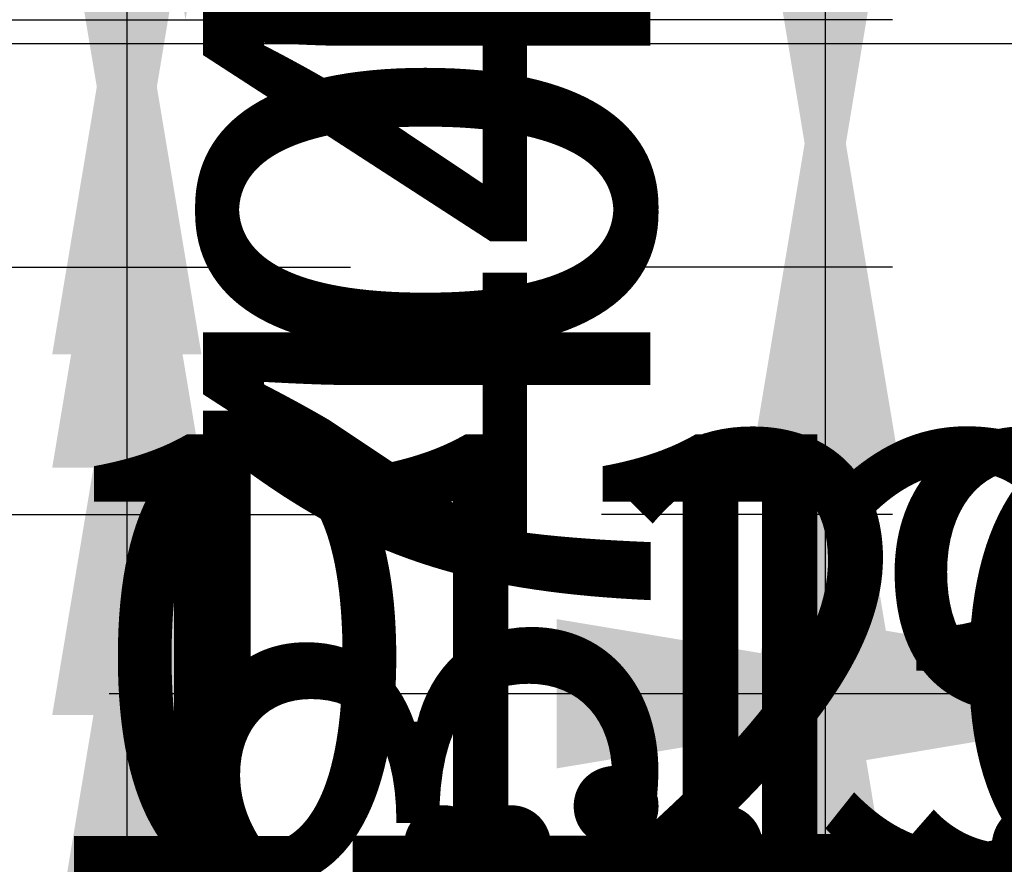
# Model space of a CAD drawing. Units: metres. Extents: x 782 to 1487, y 1262 to 7446.
# Tile 12 of 25: x 834.592 to 840.091, y 1288.353 to 1293.067. Entities that reach past the tile are written whole.
import ezdxf

# ---------------------------------------------------------------- set-up
doc = ezdxf.new("R2010")
doc.units = ezdxf.units.M
doc.layers.add('A-ANNO-DIMS', color=2, linetype='Continuous', lineweight=18)
doc.styles.get("Standard").update_dxf_attribs({"font": 'arial.ttf'})
doc.dimstyles.new('ISO-25', dxfattribs={"dimtxt": 2.5, "dimasz": 2.5, "dimexe": 1.25, "dimexo": 0.625, "dimtad": 1, "dimtxsty": 'Standard', "dimcen": 2.5, "dimadec": 0, "dimazin": 0, "dimtfac": 1, "dimtmove": 0, "dimatfit": 3, "dimfxl": 1, "dimarcsym": 0})

# ---------------------------------------------------------------- blocks, each defined once
blk = doc.blocks.new('*D6')
at = {"layer": 'A-ANNO-DIMS', "color": 0, "lineweight": -2, "transparency": 16777216}
for p, q in [((833.0375, 1307.3274), (836.7683, 1307.3274)), ((835.5183, 1304.8274), (835.5183, 1295.5674)), ((833.0375, 1293.0674), (836.7683, 1293.0674))]:
    blk.add_line(p, q, dxfattribs=at)
at = {"layer": 'A-ANNO-DIMS', "color": 0, "transparency": 16777216}
for points in [[(835.1017, 1304.8274), (835.935, 1304.8274), (835.5183, 1307.3274)], [(835.1017, 1295.5674), (835.935, 1295.5674), (835.5183, 1293.0674)]]:
    blk.add_solid(points, dxfattribs=at)
at = {"layer": 'Defpoints', "color": 0, "transparency": 16777216}
for p in [(832.4125, 1307.3274), (832.4125, 1293.0674), (835.5183, 1293.0674)]:
    blk.add_point(p, dxfattribs=at)
at = {"layer": 'A-ANNO-DIMS', "color": 0, "transparency": 16777216, "insert": (833.3909, 1300.1974), "char_height": 2.5, "attachment_point": 5, "rotation": 90}
blk.add_mtext('14,26', dxfattribs=at)
blk = doc.blocks.new('*D22')
at = {"layer": 'A-ANNO-DIMS', "color": 0, "lineweight": -2, "transparency": 16777216}
for p, q in [((812.7897, 1292.934), (810.2897, 1292.934)), ((815.2897, 1292.934), (816.1792, 1292.934)), ((818.6792, 1292.934), (848.8344, 1292.934)), ((815.2897, 1292.4424), (815.2897, 1291.684)), ((816.1792, 1292.4424), (816.1792, 1291.684))]:
    blk.add_line(p, q, dxfattribs=at)
at = {"layer": 'A-ANNO-DIMS', "color": 0, "transparency": 16777216}
for points in [[(812.7897, 1293.3507), (812.7897, 1292.5173), (815.2897, 1292.934)], [(818.6792, 1293.3507), (818.6792, 1292.5173), (816.1792, 1292.934)]]:
    blk.add_solid(points, dxfattribs=at)
at = {"layer": 'Defpoints', "color": 0, "transparency": 16777216}
for p in [(815.2897, 1293.0674), (816.1792, 1293.0674), (816.1792, 1292.934)]:
    blk.add_point(p, dxfattribs=at)
at = {"layer": 'A-ANNO-DIMS', "color": 0, "transparency": 16777216, "insert": (835.0068, 1294.8525), "char_height": 2.5, "attachment_point": 5}
blk.add_mtext('DOOR 0.89 TYP.', dxfattribs=at)
blk = doc.blocks.new('*D24')
at = {"layer": 'A-ANNO-DIMS', "color": 0, "lineweight": -2, "transparency": 16777216}
for p, q in [((811.2086, 1294.4231), (808.7086, 1294.4231)), ((813.7086, 1294.4231), (814.5592, 1294.4231)), ((817.0592, 1294.4231), (852.6493, 1294.4231)), ((813.7086, 1293.9257), (813.7086, 1293.1731)), ((814.5592, 1293.9257), (814.5592, 1293.1731))]:
    blk.add_line(p, q, dxfattribs=at)
at = {"layer": 'A-ANNO-DIMS', "color": 0, "transparency": 16777216}
for points in [[(811.2086, 1294.8398), (811.2086, 1294.0065), (813.7086, 1294.4231)], [(817.0592, 1294.8398), (817.0592, 1294.0065), (814.5592, 1294.4231)]]:
    blk.add_solid(points, dxfattribs=at)
at = {"layer": 'Defpoints', "color": 0, "transparency": 16777216}
for p in [(813.7086, 1294.5507), (814.5592, 1294.5507), (814.5592, 1294.4231)]:
    blk.add_point(p, dxfattribs=at)
at = {"layer": 'A-ANNO-DIMS', "color": 0, "transparency": 16777216, "insert": (836.1042, 1296.3416), "char_height": 2.5, "attachment_point": 5}
blk.add_mtext('DOOR D2 0.85 TYP.', dxfattribs=at)
blk = doc.blocks.new('*D87')
at = {"layer": 'A-ANNO-DIMS', "color": 0, "lineweight": -2, "transparency": 16777216}
for p, q in [((835.1905, 1309.8274), (835.1905, 1312.3274)), ((833.0375, 1307.3274), (836.4405, 1307.3274)), ((835.1905, 1307.3274), (835.1905, 1304.8669)), ((833.0382, 1304.8669), (836.4405, 1304.8669)), ((835.1905, 1302.3669), (835.1905, 1292.0821))]:
    blk.add_line(p, q, dxfattribs=at)
at = {"layer": 'A-ANNO-DIMS', "color": 0, "transparency": 16777216}
for points in [[(834.7738, 1309.8274), (835.6071, 1309.8274), (835.1905, 1307.3274)], [(834.7738, 1302.3669), (835.6071, 1302.3669), (835.1905, 1304.8669)]]:
    blk.add_solid(points, dxfattribs=at)
at = {"layer": 'Defpoints', "color": 0, "transparency": 16777216}
for p in [(832.4125, 1307.3274), (832.4132, 1304.8669), (835.1905, 1304.8669)]:
    blk.add_point(p, dxfattribs=at)
at = {"layer": 'A-ANNO-DIMS', "color": 0, "transparency": 16777216, "insert": (833.289, 1295.9745), "char_height": 2.5, "attachment_point": 5, "rotation": 90}
blk.add_mtext('2.46', dxfattribs=at)
blk = doc.blocks.new('*D88')
at = {"layer": 'A-ANNO-DIMS', "color": 0, "lineweight": -2, "transparency": 16777216}
for p, q in [((835.1905, 1307.3669), (835.1905, 1309.8669)), ((833.0382, 1304.8669), (836.4405, 1304.8669)), ((835.1905, 1304.8669), (835.1905, 1300.3378)), ((833.0381, 1300.3378), (836.4405, 1300.3378)), ((835.1905, 1297.8378), (835.1905, 1285.5459))]:
    blk.add_line(p, q, dxfattribs=at)
at = {"layer": 'A-ANNO-DIMS', "color": 0, "transparency": 16777216}
for points in [[(834.7738, 1307.3669), (835.6071, 1307.3669), (835.1905, 1304.8669)], [(834.7738, 1297.8378), (835.6071, 1297.8378), (835.1905, 1300.3378)]]:
    blk.add_solid(points, dxfattribs=at)
at = {"layer": 'Defpoints', "color": 0, "transparency": 16777216}
for p in [(832.4132, 1304.8669), (832.4131, 1300.3378), (835.1905, 1300.3378)]:
    blk.add_point(p, dxfattribs=at)
at = {"layer": 'A-ANNO-DIMS', "color": 0, "transparency": 16777216, "insert": (833.289, 1290.4419), "char_height": 2.5, "attachment_point": 5, "rotation": 90}
blk.add_mtext('4.529', dxfattribs=at)
blk = doc.blocks.new('*D89')
at = {"layer": 'A-ANNO-DIMS', "color": 0, "lineweight": -2, "transparency": 16777216}
for p, q in [((835.1905, 1302.8378), (835.1905, 1305.3378)), ((833.0381, 1300.3378), (836.4405, 1300.3378)), ((835.1905, 1300.3378), (835.1905, 1296.196)), ((833.0375, 1296.196), (836.4405, 1296.196)), ((835.1905, 1293.696), (835.1905, 1281.4347))]:
    blk.add_line(p, q, dxfattribs=at)
at = {"layer": 'A-ANNO-DIMS', "color": 0, "transparency": 16777216}
for points in [[(834.7738, 1302.8378), (835.6071, 1302.8378), (835.1905, 1300.3378)], [(834.7738, 1293.696), (835.6071, 1293.696), (835.1905, 1296.196)]]:
    blk.add_solid(points, dxfattribs=at)
at = {"layer": 'Defpoints', "color": 0, "transparency": 16777216}
for p in [(832.4131, 1300.3378), (832.4125, 1296.196), (835.1905, 1296.196)]:
    blk.add_point(p, dxfattribs=at)
at = {"layer": 'A-ANNO-DIMS', "color": 0, "transparency": 16777216, "insert": (833.3103, 1286.3153), "char_height": 2.5, "attachment_point": 5, "rotation": 90}
blk.add_mtext('4.142', dxfattribs=at)
blk = doc.blocks.new('*D90')
at = {"layer": 'A-ANNO-DIMS', "color": 0, "lineweight": -2, "transparency": 16777216}
for p, q in [((835.1905, 1298.696), (835.1905, 1301.196)), ((833.0375, 1296.196), (836.4405, 1296.196)), ((835.1905, 1296.196), (835.1905, 1293.6994)), ((833.0375, 1293.6994), (836.4405, 1293.6994)), ((835.1905, 1291.1994), (835.1905, 1280.9214))]:
    blk.add_line(p, q, dxfattribs=at)
at = {"layer": 'A-ANNO-DIMS', "color": 0, "transparency": 16777216}
for points in [[(834.7738, 1298.696), (835.6071, 1298.696), (835.1905, 1296.196)], [(834.7738, 1291.1994), (835.6071, 1291.1994), (835.1905, 1293.6994)]]:
    blk.add_solid(points, dxfattribs=at)
at = {"layer": 'Defpoints', "color": 0, "transparency": 16777216}
for p in [(832.4125, 1296.196), (832.4125, 1293.6994), (835.1905, 1293.6994)]:
    blk.add_point(p, dxfattribs=at)
at = {"layer": 'A-ANNO-DIMS', "color": 0, "transparency": 16777216, "insert": (833.289, 1284.8104), "char_height": 2.5, "attachment_point": 5, "rotation": 90}
blk.add_mtext('2.50', dxfattribs=at)
blk = doc.blocks.new('*D91')
at = {"layer": 'A-ANNO-DIMS', "color": 0, "lineweight": -2, "transparency": 16777216}
for p, q in [((835.1905, 1296.1994), (835.1905, 1298.6994)), ((833.0375, 1293.6994), (836.4405, 1293.6994)), ((835.1905, 1293.6994), (835.1905, 1293.0674)), ((833.0375, 1293.0674), (836.4405, 1293.0674)), ((835.1905, 1290.5674), (835.1905, 1278.4068))]:
    blk.add_line(p, q, dxfattribs=at)
at = {"layer": 'A-ANNO-DIMS', "color": 0, "transparency": 16777216}
for points in [[(834.7738, 1296.1994), (835.6071, 1296.1994), (835.1905, 1293.6994)], [(834.7738, 1290.5674), (835.6071, 1290.5674), (835.1905, 1293.0674)]]:
    blk.add_solid(points, dxfattribs=at)
at = {"layer": 'Defpoints', "color": 0, "transparency": 16777216}
for p in [(832.4125, 1293.6994), (832.4125, 1293.0674), (835.1905, 1293.0674)]:
    blk.add_point(p, dxfattribs=at)
at = {"layer": 'A-ANNO-DIMS', "color": 0, "transparency": 16777216, "insert": (833.2882, 1283.2371), "char_height": 2.5, "attachment_point": 5, "rotation": 90}
blk.add_mtext('0.632', dxfattribs=at)
blk = doc.blocks.new('*D92')
at = {"layer": 'A-ANNO-DIMS', "color": 0, "lineweight": -2, "transparency": 16777216}
for p, q in [((835.1905, 1295.5674), (835.1905, 1298.0674)), ((831.3406, 1293.0674), (836.4405, 1293.0674)), ((835.1905, 1293.0674), (835.1905, 1291.6863)), ((831.3406, 1291.6863), (836.4405, 1291.6863)), ((835.1905, 1289.1863), (835.1905, 1277.7181))]:
    blk.add_line(p, q, dxfattribs=at)
at = {"layer": 'A-ANNO-DIMS', "color": 0, "transparency": 16777216}
for points in [[(834.7738, 1295.5674), (835.6071, 1295.5674), (835.1905, 1293.0674)], [(834.7738, 1289.1863), (835.6071, 1289.1863), (835.1905, 1291.6863)]]:
    blk.add_solid(points, dxfattribs=at)
at = {"layer": 'Defpoints', "color": 0, "transparency": 16777216}
for p in [(830.7156, 1293.0674), (830.7156, 1291.6863), (835.1905, 1291.6863)]:
    blk.add_point(p, dxfattribs=at)
at = {"layer": 'A-ANNO-DIMS', "color": 0, "transparency": 16777216, "insert": (833.2882, 1282.2022), "char_height": 2.5, "attachment_point": 5, "rotation": 90}
blk.add_mtext('1.381', dxfattribs=at)
blk = doc.blocks.new('*D93')
at = {"layer": 'A-ANNO-DIMS', "color": 0, "lineweight": -2, "transparency": 16777216}
for p, q in [((835.1905, 1294.1863), (835.1905, 1296.6863)), ((831.3406, 1291.6863), (836.4405, 1291.6863)), ((835.1905, 1291.6863), (835.1905, 1290.3053)), ((831.3406, 1290.3053), (836.4405, 1290.3053)), ((835.1905, 1287.8053), (835.1905, 1276.337))]:
    blk.add_line(p, q, dxfattribs=at)
at = {"layer": 'A-ANNO-DIMS', "color": 0, "transparency": 16777216}
for points in [[(834.7738, 1294.1863), (835.6071, 1294.1863), (835.1905, 1291.6863)], [(834.7738, 1287.8053), (835.6071, 1287.8053), (835.1905, 1290.3053)]]:
    blk.add_solid(points, dxfattribs=at)
at = {"layer": 'Defpoints', "color": 0, "transparency": 16777216}
for p in [(830.7156, 1291.6863), (830.7156, 1290.3053), (835.1905, 1290.3053)]:
    blk.add_point(p, dxfattribs=at)
at = {"layer": 'A-ANNO-DIMS', "color": 0, "transparency": 16777216, "insert": (833.2882, 1280.8211), "char_height": 2.5, "attachment_point": 5, "rotation": 90}
blk.add_mtext('1.381', dxfattribs=at)
blk = doc.blocks.new('*D97')
at = {"layer": 'A-ANNO-DIMS', "color": 0, "lineweight": -2, "transparency": 16777216}
for p, q in [((827.9625, 1289.6803), (827.9625, 1286.0275)), ((829.1513, 1289.6803), (829.1513, 1286.0275)), ((825.4625, 1287.2775), (822.9625, 1287.2775)), ((827.9625, 1287.2775), (829.1513, 1287.2775)), ((831.6513, 1287.2775), (841.6649, 1287.2775))]:
    blk.add_line(p, q, dxfattribs=at)
at = {"layer": 'A-ANNO-DIMS', "color": 0, "transparency": 16777216}
for points in [[(825.4625, 1287.6941), (825.4625, 1286.8608), (827.9625, 1287.2775)], [(831.6513, 1287.6941), (831.6513, 1286.8608), (829.1513, 1287.2775)]]:
    blk.add_solid(points, dxfattribs=at)
at = {"layer": 'Defpoints', "color": 0, "transparency": 16777216}
for p in [(827.9625, 1290.3053), (829.1513, 1290.3053), (829.1513, 1287.2775)]:
    blk.add_point(p, dxfattribs=at)
at = {"layer": 'A-ANNO-DIMS', "color": 0, "transparency": 16777216, "insert": (837.9081, 1289.1789), "char_height": 2.5, "attachment_point": 5}
blk.add_mtext('1.19', dxfattribs=at)
blk = doc.blocks.new('*D98')
at = {"layer": 'A-ANNO-DIMS', "color": 0, "lineweight": -2, "transparency": 16777216}
for p, q in [((829.1513, 1289.6803), (829.1513, 1286.0275)), ((829.412, 1289.6803), (829.412, 1286.0275)), ((826.6513, 1287.2775), (824.1513, 1287.2775)), ((829.1513, 1287.2775), (829.412, 1287.2775)), ((831.912, 1287.2775), (842.1542, 1287.2775))]:
    blk.add_line(p, q, dxfattribs=at)
at = {"layer": 'A-ANNO-DIMS', "color": 0, "transparency": 16777216}
for points in [[(826.6513, 1287.6941), (826.6513, 1286.8608), (829.1513, 1287.2775)], [(831.912, 1287.6941), (831.912, 1286.8608), (829.412, 1287.2775)]]:
    blk.add_solid(points, dxfattribs=at)
at = {"layer": 'Defpoints', "color": 0, "transparency": 16777216}
for p in [(829.1513, 1290.3053), (829.412, 1290.3053), (829.412, 1287.2775)]:
    blk.add_point(p, dxfattribs=at)
at = {"layer": 'A-ANNO-DIMS', "color": 0, "transparency": 16777216, "insert": (838.2831, 1289.1789), "char_height": 2.5, "attachment_point": 5}
blk.add_mtext('0.26', dxfattribs=at)
blk = doc.blocks.new('*D99')
at = {"layer": 'A-ANNO-DIMS', "color": 0, "lineweight": -2, "transparency": 16777216}
for p, q in [((829.412, 1289.6803), (829.412, 1286.0275)), ((830.7156, 1289.6803), (830.7156, 1286.0275)), ((826.912, 1287.2775), (824.412, 1287.2775)), ((829.412, 1287.2775), (830.7156, 1287.2775)), ((833.2156, 1287.2775), (843.2156, 1287.2775))]:
    blk.add_line(p, q, dxfattribs=at)
at = {"layer": 'A-ANNO-DIMS', "color": 0, "transparency": 16777216}
for points in [[(826.912, 1287.6941), (826.912, 1286.8608), (829.412, 1287.2775)], [(833.2156, 1287.6941), (833.2156, 1286.8608), (830.7156, 1287.2775)]]:
    blk.add_solid(points, dxfattribs=at)
at = {"layer": 'Defpoints', "color": 0, "transparency": 16777216}
for p in [(829.412, 1290.3053), (830.7156, 1290.3053), (830.7156, 1287.2775)]:
    blk.add_point(p, dxfattribs=at)
at = {"layer": 'A-ANNO-DIMS', "color": 0, "transparency": 16777216, "insert": (839.4656, 1289.1798), "char_height": 2.5, "attachment_point": 5}
blk.add_mtext('1.30', dxfattribs=at)
blk = doc.blocks.new('*D100')
at = {"layer": 'A-ANNO-DIMS', "color": 0, "lineweight": -2, "transparency": 16777216}
for p, q in [((830.7156, 1289.6803), (830.7156, 1286.0275)), ((832.4125, 1289.6803), (832.4125, 1286.0275)), ((828.2156, 1287.2775), (825.7156, 1287.2775)), ((830.7156, 1287.2775), (832.4125, 1287.2775)), ((834.9125, 1287.2775), (846.8634, 1287.2775))]:
    blk.add_line(p, q, dxfattribs=at)
at = {"layer": 'A-ANNO-DIMS', "color": 0, "transparency": 16777216}
for points in [[(828.2156, 1287.6941), (828.2156, 1286.8608), (830.7156, 1287.2775)], [(834.9125, 1287.6941), (834.9125, 1286.8608), (832.4125, 1287.2775)]]:
    blk.add_solid(points, dxfattribs=at)
at = {"layer": 'Defpoints', "color": 0, "transparency": 16777216}
for p in [(830.7156, 1290.3053), (832.4125, 1290.3053), (832.4125, 1287.2775)]:
    blk.add_point(p, dxfattribs=at)
at = {"layer": 'A-ANNO-DIMS', "color": 0, "transparency": 16777216, "insert": (842.1379, 1289.1789), "char_height": 2.5, "attachment_point": 5}
blk.add_mtext('1.697', dxfattribs=at)
blk = doc.blocks.new('*D105')
at = {"layer": 'A-ANNO-DIMS', "color": 0, "lineweight": -2, "transparency": 16777216}
for p, q in [((840.0913, 1289.6803), (840.0913, 1288.0553)), ((841.2801, 1289.6803), (841.2801, 1288.0553)), ((837.5913, 1289.3053), (835.0913, 1289.3053)), ((840.0913, 1289.3053), (841.2801, 1289.3053)), ((843.7801, 1289.3053), (853.7938, 1289.3053))]:
    blk.add_line(p, q, dxfattribs=at)
at = {"layer": 'A-ANNO-DIMS', "color": 0, "transparency": 16777216}
for points in [[(837.5913, 1289.7219), (837.5913, 1288.8886), (840.0913, 1289.3053)], [(843.7801, 1289.7219), (843.7801, 1288.8886), (841.2801, 1289.3053)]]:
    blk.add_solid(points, dxfattribs=at)
at = {"layer": 'Defpoints', "color": 0, "transparency": 16777216}
for p in [(840.0913, 1290.3053), (841.2801, 1290.3053), (841.2801, 1289.3053)]:
    blk.add_point(p, dxfattribs=at)
at = {"layer": 'A-ANNO-DIMS', "color": 0, "transparency": 16777216, "insert": (850.037, 1291.2067), "char_height": 2.5, "attachment_point": 5}
blk.add_mtext('1.19', dxfattribs=at)
blk = doc.blocks.new('*D106')
at = {"layer": 'A-ANNO-DIMS', "color": 0, "lineweight": -2, "transparency": 16777216}
for p, q in [((841.2801, 1289.6803), (841.2801, 1288.0553)), ((841.5409, 1289.6803), (841.5409, 1288.0553)), ((838.7801, 1289.3053), (836.2801, 1289.3053)), ((841.2801, 1289.3053), (841.5409, 1289.3053)), ((844.0409, 1289.3053), (854.283, 1289.3053))]:
    blk.add_line(p, q, dxfattribs=at)
at = {"layer": 'A-ANNO-DIMS', "color": 0, "transparency": 16777216}
for points in [[(838.7801, 1289.7219), (838.7801, 1288.8886), (841.2801, 1289.3053)], [(844.0409, 1289.7219), (844.0409, 1288.8886), (841.5409, 1289.3053)]]:
    blk.add_solid(points, dxfattribs=at)
at = {"layer": 'Defpoints', "color": 0, "transparency": 16777216}
for p in [(841.2801, 1290.3053), (841.5409, 1290.3053), (841.5409, 1289.3053)]:
    blk.add_point(p, dxfattribs=at)
at = {"layer": 'A-ANNO-DIMS', "color": 0, "transparency": 16777216, "insert": (850.4119, 1291.2067), "char_height": 2.5, "attachment_point": 5}
blk.add_mtext('0.26', dxfattribs=at)
blk = doc.blocks.new('*D107')
at = {"layer": 'A-ANNO-DIMS', "color": 0, "lineweight": -2, "transparency": 16777216}
for p, q in [((841.5409, 1289.6803), (841.5409, 1288.0553)), ((842.8445, 1289.6803), (842.8445, 1288.0553)), ((839.0409, 1289.3053), (836.5409, 1289.3053)), ((841.5409, 1289.3053), (842.8445, 1289.3053)), ((845.3445, 1289.3053), (855.3445, 1289.3053))]:
    blk.add_line(p, q, dxfattribs=at)
at = {"layer": 'A-ANNO-DIMS', "color": 0, "transparency": 16777216}
for points in [[(839.0409, 1289.7219), (839.0409, 1288.8886), (841.5409, 1289.3053)], [(845.3445, 1289.7219), (845.3445, 1288.8886), (842.8445, 1289.3053)]]:
    blk.add_solid(points, dxfattribs=at)
at = {"layer": 'Defpoints', "color": 0, "transparency": 16777216}
for p in [(841.5409, 1290.3053), (842.8445, 1290.3053), (842.8445, 1289.3053)]:
    blk.add_point(p, dxfattribs=at)
at = {"layer": 'A-ANNO-DIMS', "color": 0, "transparency": 16777216, "insert": (851.5945, 1291.2076), "char_height": 2.5, "attachment_point": 5}
blk.add_mtext('1.30', dxfattribs=at)
blk = doc.blocks.new('*D108')
at = {"layer": 'A-ANNO-DIMS', "color": 0, "lineweight": -2, "transparency": 16777216}
for p, q in [((842.8445, 1289.6803), (842.8445, 1288.0553)), ((844.1849, 1289.6803), (844.1849, 1288.0553)), ((840.3445, 1289.3053), (837.8445, 1289.3053)), ((842.8445, 1289.3053), (844.1849, 1289.3053)), ((846.6849, 1289.3053), (856.6832, 1289.3053))]:
    blk.add_line(p, q, dxfattribs=at)
at = {"layer": 'A-ANNO-DIMS', "color": 0, "transparency": 16777216}
for points in [[(840.3445, 1289.7219), (840.3445, 1288.8886), (842.8445, 1289.3053)], [(846.6849, 1289.7219), (846.6849, 1288.8886), (844.1849, 1289.3053)]]:
    blk.add_solid(points, dxfattribs=at)
at = {"layer": 'Defpoints', "color": 0, "transparency": 16777216}
for p in [(842.8445, 1290.3053), (844.1849, 1290.3053), (844.1849, 1289.3053)]:
    blk.add_point(p, dxfattribs=at)
at = {"layer": 'A-ANNO-DIMS', "color": 0, "transparency": 16777216, "insert": (852.934, 1291.2076), "char_height": 2.5, "attachment_point": 5}
blk.add_mtext('1.34', dxfattribs=at)
blk = doc.blocks.new('*D109')
at = {"layer": 'A-ANNO-DIMS', "color": 0, "lineweight": -2, "transparency": 16777216}
for p, q in [((839.0913, 1308.3353), (839.0913, 1310.8353)), ((839.4663, 1305.8353), (837.8413, 1305.8353)), ((839.0913, 1305.8353), (839.0913, 1305.1633)), ((839.4663, 1305.1633), (837.8413, 1305.1633)), ((839.0913, 1302.6633), (839.0913, 1290.5026))]:
    blk.add_line(p, q, dxfattribs=at)
at = {"layer": 'A-ANNO-DIMS', "color": 0, "transparency": 16777216}
for points in [[(838.6746, 1308.3353), (839.508, 1308.3353), (839.0913, 1305.8353)], [(838.6746, 1302.6633), (839.508, 1302.6633), (839.0913, 1305.1633)]]:
    blk.add_solid(points, dxfattribs=at)
at = {"layer": 'Defpoints', "color": 0, "transparency": 16777216}
for p in [(840.0913, 1305.8353), (839.0913, 1305.1633), (840.0913, 1305.1633)]:
    blk.add_point(p, dxfattribs=at)
at = {"layer": 'A-ANNO-DIMS', "color": 0, "transparency": 16777216, "insert": (837.1899, 1295.333), "char_height": 2.5, "attachment_point": 5, "rotation": 90}
blk.add_mtext('0.672', dxfattribs=at)
blk = doc.blocks.new('*D110')
at = {"layer": 'A-ANNO-DIMS', "color": 0, "lineweight": -2, "transparency": 16777216}
for p, q in [((839.0913, 1307.6633), (839.0913, 1310.1633)), ((839.4663, 1305.1633), (837.8413, 1305.1633)), ((839.0913, 1305.1633), (839.0913, 1300.4593)), ((839.4663, 1300.4593), (837.8413, 1300.4593)), ((839.0913, 1297.9593), (839.0913, 1285.6827))]:
    blk.add_line(p, q, dxfattribs=at)
at = {"layer": 'A-ANNO-DIMS', "color": 0, "transparency": 16777216}
for points in [[(838.6746, 1307.6633), (839.508, 1307.6633), (839.0913, 1305.1633)], [(838.6746, 1297.9593), (839.508, 1297.9593), (839.0913, 1300.4593)]]:
    blk.add_solid(points, dxfattribs=at)
at = {"layer": 'Defpoints', "color": 0, "transparency": 16777216}
for p in [(840.0913, 1305.1633), (839.0913, 1300.4593), (840.0913, 1300.4593)]:
    blk.add_point(p, dxfattribs=at)
at = {"layer": 'A-ANNO-DIMS', "color": 0, "transparency": 16777216, "insert": (837.1899, 1290.571), "char_height": 2.5, "attachment_point": 5, "rotation": 90}
blk.add_mtext('4.704', dxfattribs=at)
blk = doc.blocks.new('*D111')
at = {"layer": 'A-ANNO-DIMS', "color": 0, "lineweight": -2, "transparency": 16777216}
for p, q in [((839.0913, 1302.9593), (839.0913, 1305.4593)), ((839.4663, 1300.4593), (837.8413, 1300.4593)), ((839.0913, 1300.4593), (839.0913, 1299.1153)), ((839.4663, 1299.1153), (837.8413, 1299.1153)), ((839.0913, 1296.6153), (839.0913, 1284.6747))]:
    blk.add_line(p, q, dxfattribs=at)
at = {"layer": 'A-ANNO-DIMS', "color": 0, "transparency": 16777216}
for points in [[(838.6746, 1302.9593), (839.508, 1302.9593), (839.0913, 1300.4593)], [(838.6746, 1296.6153), (839.508, 1296.6153), (839.0913, 1299.1153)]]:
    blk.add_solid(points, dxfattribs=at)
at = {"layer": 'Defpoints', "color": 0, "transparency": 16777216}
for p in [(840.0913, 1300.4593), (839.0913, 1299.1153), (840.0913, 1299.1153)]:
    blk.add_point(p, dxfattribs=at)
at = {"layer": 'A-ANNO-DIMS', "color": 0, "transparency": 16777216, "insert": (837.189, 1289.395), "char_height": 2.5, "attachment_point": 5, "rotation": 90}
blk.add_mtext('1.344', dxfattribs=at)
blk = doc.blocks.new('*D112')
at = {"layer": 'A-ANNO-DIMS', "color": 0, "lineweight": -2, "transparency": 16777216}
for p, q in [((839.0913, 1301.6153), (839.0913, 1304.1153)), ((839.4663, 1299.1153), (837.8413, 1299.1153)), ((839.0913, 1299.1153), (839.0913, 1293.0674)), ((839.4663, 1293.0674), (837.8413, 1293.0674)), ((839.0913, 1290.5674), (839.0913, 1278.3624))]:
    blk.add_line(p, q, dxfattribs=at)
at = {"layer": 'A-ANNO-DIMS', "color": 0, "transparency": 16777216}
for points in [[(838.6746, 1301.6153), (839.508, 1301.6153), (839.0913, 1299.1153)], [(838.6746, 1290.5674), (839.508, 1290.5674), (839.0913, 1293.0674)]]:
    blk.add_solid(points, dxfattribs=at)
at = {"layer": 'Defpoints', "color": 0, "transparency": 16777216}
for p in [(840.0913, 1299.1153), (839.0913, 1293.0674), (840.0913, 1293.0674)]:
    blk.add_point(p, dxfattribs=at)
at = {"layer": 'A-ANNO-DIMS', "color": 0, "transparency": 16777216, "insert": (837.1899, 1283.2149), "char_height": 2.5, "attachment_point": 5, "rotation": 90}
blk.add_mtext('6.048', dxfattribs=at)
blk = doc.blocks.new('*D113')
at = {"layer": 'A-ANNO-DIMS', "color": 0, "lineweight": -2, "transparency": 16777216}
for p, q in [((839.0913, 1295.5674), (839.0913, 1298.0674)), ((839.4663, 1293.0674), (837.8413, 1293.0674)), ((839.0913, 1293.0674), (839.0913, 1291.6863)), ((839.4663, 1291.6863), (837.8413, 1291.6863)), ((839.0913, 1289.1863), (839.0913, 1277.7181))]:
    blk.add_line(p, q, dxfattribs=at)
at = {"layer": 'A-ANNO-DIMS', "color": 0, "transparency": 16777216}
for points in [[(838.6746, 1295.5674), (839.508, 1295.5674), (839.0913, 1293.0674)], [(838.6746, 1289.1863), (839.508, 1289.1863), (839.0913, 1291.6863)]]:
    blk.add_solid(points, dxfattribs=at)
at = {"layer": 'Defpoints', "color": 0, "transparency": 16777216}
for p in [(840.0913, 1293.0674), (839.0913, 1291.6863), (840.0913, 1291.6863)]:
    blk.add_point(p, dxfattribs=at)
at = {"layer": 'A-ANNO-DIMS', "color": 0, "transparency": 16777216, "insert": (837.189, 1282.2022), "char_height": 2.5, "attachment_point": 5, "rotation": 90}
blk.add_mtext('1.381', dxfattribs=at)
blk = doc.blocks.new('*D114')
at = {"layer": 'A-ANNO-DIMS', "color": 0, "lineweight": -2, "transparency": 16777216}
for p, q in [((839.0913, 1294.1863), (839.0913, 1296.6863)), ((839.4663, 1291.6863), (837.8413, 1291.6863)), ((839.0913, 1291.6863), (839.0913, 1290.3053)), ((839.4663, 1290.3053), (837.8413, 1290.3053)), ((839.0913, 1287.8053), (839.0913, 1276.337))]:
    blk.add_line(p, q, dxfattribs=at)
at = {"layer": 'A-ANNO-DIMS', "color": 0, "transparency": 16777216}
for points in [[(838.6746, 1294.1863), (839.508, 1294.1863), (839.0913, 1291.6863)], [(838.6746, 1287.8053), (839.508, 1287.8053), (839.0913, 1290.3053)]]:
    blk.add_solid(points, dxfattribs=at)
at = {"layer": 'Defpoints', "color": 0, "transparency": 16777216}
for p in [(840.0913, 1291.6863), (839.0913, 1290.3053), (840.0913, 1290.3053)]:
    blk.add_point(p, dxfattribs=at)
at = {"layer": 'A-ANNO-DIMS', "color": 0, "transparency": 16777216, "insert": (837.189, 1280.8211), "char_height": 2.5, "attachment_point": 5, "rotation": 90}
blk.add_mtext('1.381', dxfattribs=at)
blk = doc.blocks.new('*D157')
at = {"layer": 'A-ANNO-DIMS', "color": 0, "lineweight": -2, "transparency": 16777216}
for p, q in [((834.2886, 1282.619), (834.2886, 1294.8189)), ((835.8783, 1282.619), (833.0386, 1282.619)), ((834.2886, 1278.7022), (834.2886, 1280.119)), ((835.8783, 1276.2022), (833.0386, 1276.2022))]:
    blk.add_line(p, q, dxfattribs=at)
at = {"layer": 'A-ANNO-DIMS', "color": 0, "transparency": 16777216}
for points in [[(833.8719, 1280.119), (834.7052, 1280.119), (834.2886, 1282.619)], [(833.8719, 1278.7022), (834.7052, 1278.7022), (834.2886, 1276.2022)]]:
    blk.add_solid(points, dxfattribs=at)
at = {"layer": 'Defpoints', "color": 0, "transparency": 16777216}
for p in [(834.2886, 1282.619), (836.5033, 1282.619), (836.5033, 1276.2022)]:
    blk.add_point(p, dxfattribs=at)
at = {"layer": 'A-ANNO-DIMS', "color": 0, "transparency": 16777216, "insert": (832.3871, 1289.9689), "char_height": 2.5, "attachment_point": 5, "rotation": 90}
blk.add_mtext('6.417', dxfattribs=at)

msp = doc.modelspace()

# ---------------------------------------------------------------- dimensions: what is measured, and where the dimension line sits
at = {"layer": 'A-ANNO-DIMS'}
for base, p1, p2, override, picture, middle in [((835.1905, 1304.8669), (832.4125, 1307.3274), (832.4132, 1304.8669), {"dimdec": 2, "dimlfac": 1, "dimrnd": 0, "dimzin": 0, "dimdsep": 46, "dimlunit": 2}, '*D87', (833.289, 1295.9745)), ((839.0913, 1305.1633), (840.0913, 1305.8353), (840.0913, 1305.1633), {"dimdec": 3, "dimlfac": 1, "dimrnd": 0, "dimzin": 0, "dimdsep": 46, "dimlunit": 2}, '*D109', (837.1899, 1295.333)), ((839.0913, 1300.4593), (840.0913, 1305.1633), (840.0913, 1300.4593), {"dimdec": 3, "dimlfac": 1, "dimrnd": 0, "dimzin": 0, "dimdsep": 46, "dimlunit": 2}, '*D110', (837.1899, 1290.571)), ((835.1905, 1300.3378), (832.4132, 1304.8669), (832.4131, 1300.3378), {"dimdec": 3, "dimlfac": 1, "dimrnd": 0, "dimzin": 0, "dimdsep": 46, "dimlunit": 2}, '*D88', (833.289, 1290.4419)), ((835.5183, 1293.0674), (832.4125, 1307.3274), (832.4125, 1293.0674), {"dimclrd": 0, "dimclre": 0, "dimclrt": 0}, '*D6', (833.3909, 1300.1974)), ((839.0913, 1299.1153), (840.0913, 1300.4593), (840.0913, 1299.1153), {"dimdec": 3, "dimlfac": 1, "dimrnd": 0, "dimzin": 0, "dimdsep": 46, "dimlunit": 2}, '*D111', (837.189, 1289.395)), ((835.1905, 1296.196), (832.4131, 1300.3378), (832.4125, 1296.196), {"dimdec": 3, "dimlfac": 1, "dimrnd": 0, "dimzin": 0, "dimdsep": 46, "dimlunit": 2}, '*D89', (833.3103, 1286.3153)), ((839.0913, 1293.0674), (840.0913, 1299.1153), (840.0913, 1293.0674), {"dimdec": 3, "dimlfac": 1, "dimrnd": 0, "dimzin": 0, "dimdsep": 46, "dimlunit": 2}, '*D112', (837.1899, 1283.2149)), ((835.1905, 1293.6994), (832.4125, 1296.196), (832.4125, 1293.6994), {"dimdec": 2, "dimlfac": 1, "dimrnd": 0, "dimzin": 0, "dimdsep": 46, "dimlunit": 2}, '*D90', (833.289, 1284.8104)), ((835.1905, 1293.0674), (832.4125, 1293.6994), (832.4125, 1293.0674), {"dimdec": 3, "dimlfac": 1, "dimrnd": 0, "dimzin": 0, "dimdsep": 46, "dimlunit": 2}, '*D91', (833.2882, 1283.2371)), ((835.1905, 1291.6863), (830.7156, 1293.0674), (830.7156, 1291.6863), {"dimdec": 3, "dimlfac": 1, "dimrnd": 0, "dimzin": 0, "dimdsep": 46, "dimlunit": 2}, '*D92', (833.2882, 1282.2022)), ((839.0913, 1291.6863), (840.0913, 1293.0674), (840.0913, 1291.6863), {"dimdec": 3, "dimlfac": 1, "dimrnd": 0, "dimzin": 0, "dimdsep": 46, "dimlunit": 2}, '*D113', (837.189, 1282.2022)), ((835.1905, 1290.3053), (830.7156, 1291.6863), (830.7156, 1290.3053), {"dimdec": 3, "dimlfac": 1, "dimrnd": 0, "dimzin": 0, "dimdsep": 46, "dimlunit": 2}, '*D93', (833.2882, 1280.8211)), ((839.0913, 1290.3053), (840.0913, 1291.6863), (840.0913, 1290.3053), {"dimdec": 3, "dimlfac": 1, "dimrnd": 0, "dimzin": 0, "dimdsep": 46, "dimlunit": 2}, '*D114', (837.189, 1280.8211)), ((834.2886, 1282.619), (836.5033, 1276.2022), (836.5033, 1282.619), {"dimdec": 3, "dimlfac": 1, "dimrnd": 0, "dimzin": 0, "dimdsep": 46, "dimlunit": 2}, '*D157', (832.3871, 1289.9689))]:
    dim = msp.add_linear_dim(base=base, p1=p1, p2=p2, angle=90, dimstyle='ISO-25', override=override, dxfattribs=at)
    dim.commit()
    dim.dimension.update_dxf_attribs({"geometry": picture, "text_midpoint": middle})
for base, p1, p2, text, picture, middle in [((814.5592, 1294.4231), (813.7086, 1294.5507), (814.5592, 1294.5507), 'DOOR D2 <> TYP.', '*D24', (836.1042, 1296.3416)), ((816.1792, 1292.934), (815.2897, 1293.0674), (816.1792, 1293.0674), 'DOOR <> TYP.', '*D22', (835.0068, 1294.8525))]:
    dim = msp.add_linear_dim(base=base, p1=p1, p2=p2, text=text, dimstyle='ISO-25', override={"dimdec": 2, "dimlfac": 1, "dimrnd": 0, "dimzin": 0, "dimdsep": 46, "dimlunit": 2}, dxfattribs=at)
    dim.commit()
    dim.dimension.update_dxf_attribs({"geometry": picture, "text_midpoint": middle})
for base, p1, p2, override, picture, middle in [((841.2801, 1289.3053), (840.0913, 1290.3053), (841.2801, 1290.3053), {"dimdec": 2, "dimlfac": 1, "dimrnd": 0, "dimzin": 0, "dimdsep": 46, "dimlunit": 2}, '*D105', (850.037, 1291.2067)), ((841.5409, 1289.3053), (841.2801, 1290.3053), (841.5409, 1290.3053), {"dimdec": 2, "dimlfac": 1, "dimrnd": 0, "dimzin": 0, "dimdsep": 46, "dimlunit": 2}, '*D106', (850.4119, 1291.2067)), ((842.8445, 1289.3053), (841.5409, 1290.3053), (842.8445, 1290.3053), {"dimdec": 2, "dimlfac": 1, "dimrnd": 0, "dimzin": 0, "dimdsep": 46, "dimlunit": 2}, '*D107', (851.5945, 1291.2076)), ((844.1849, 1289.3053), (842.8445, 1290.3053), (844.1849, 1290.3053), {"dimdec": 2, "dimlfac": 1, "dimrnd": 0, "dimzin": 0, "dimdsep": 46, "dimlunit": 2}, '*D108', (852.934, 1291.2076)), ((829.1513, 1287.2775), (827.9625, 1290.3053), (829.1513, 1290.3053), {"dimdec": 2, "dimlfac": 1, "dimrnd": 0, "dimzin": 0, "dimdsep": 46, "dimlunit": 2}, '*D97', (837.9081, 1289.1789)), ((829.412, 1287.2775), (829.1513, 1290.3053), (829.412, 1290.3053), {"dimdec": 2, "dimlfac": 1, "dimrnd": 0, "dimzin": 0, "dimdsep": 46, "dimlunit": 2}, '*D98', (838.2831, 1289.1789)), ((830.7156, 1287.2775), (829.412, 1290.3053), (830.7156, 1290.3053), {"dimdec": 2, "dimlfac": 1, "dimrnd": 0, "dimzin": 0, "dimdsep": 46, "dimlunit": 2}, '*D99', (839.4656, 1289.1798)), ((832.4125, 1287.2775), (830.7156, 1290.3053), (832.4125, 1290.3053), {"dimdec": 3, "dimlfac": 1, "dimrnd": 0, "dimzin": 0, "dimdsep": 46, "dimlunit": 2}, '*D100', (842.1379, 1289.1789))]:
    dim = msp.add_linear_dim(base=base, p1=p1, p2=p2, dimstyle='ISO-25', override=override, dxfattribs=at)
    dim.commit()
    dim.dimension.update_dxf_attribs({"geometry": picture, "text_midpoint": middle})

doc.saveas('drawing.dxf')
